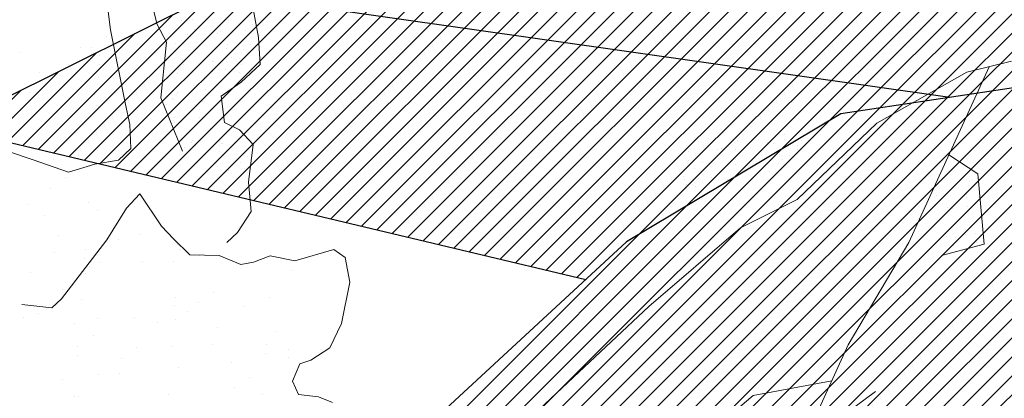
# Model space of a CAD drawing. Units: inches. Extents: x 1986 to 21484, y -1816 to 2016.
# Tile 56 of 85: x 3651.09 to 3662.33, y 1879.32 to 1883.64. Entities that reach past the tile are written whole.
import ezdxf

# ---------------------------------------------------------------- set-up
doc = ezdxf.new("R2010")
doc.units = ezdxf.units.IN
doc.layers.add('L-PLNT', color=84, linetype='Continuous', lineweight=13)
doc.layers.add('vfolhas', color=114, linetype='Continuous', lineweight=5)
doc.layers.add('vfolha2', color=110, linetype='Continuous')
doc.layers.add('vfolhas2', color=102, linetype='Continuous')
pattern_1 = [(45, (-2446.5133113, 50.986076), (-0.004419417382, 0.004419417382), [])]

# ---------------------------------------------------------------- blocks, each defined once
blk = doc.blocks.new('arbusto_PB_verde_grande')
at = {"layer": 'vfolha2'}
h = blk.add_hatch(dxfattribs=at)
h.set_pattern_fill('ANSI31', color=256, scale=0.05, style=0)
h.set_pattern_definition(pattern_1)
h.paths.add_polyline_path([(0.02944, 0.35651), (0.00028, 0.09048), (0.02625, -0.03934), (0.047, 0.06233), (0.06189, 0.09731), (0.09372, 0.26573), (0.09955, 0.43473), (0.08789, 0.61313), (0.0645, 0.72266), (0.04988, 0.6851), (0.0236, 0.51294)])
h.paths.add_polyline_path([(0.30106, 0.43789), (0.14225, 0.24871), (0.26685, 0.30022)])
h.paths.add_polyline_path([(0.37995, 0.22817), (0.23697, 0.15193), (0.18428, 0.09364), (0.11122, 0.04358), (0.02625, -0.03934), (0.28061, 0.04667), (0.36829, 0.07798), (0.46756, 0.11239), (0.61068, 0.19376), (0.71585, 0.27823), (0.55813, 0.25948)])
h.paths.add_polyline_path([(0.56101, -0.29441), (0.72752, -0.32573), (0.59024, -0.2412), (0.42962, -0.15982), (0.02625, -0.03934), (0.14922, -0.14107), (0.18838, -0.16604), (0.41501, -0.24435)])
h.paths.add_polyline_path([(-0.27429, -0.44776), (-0.30352, -0.72628), (-0.23923, -0.64175), (-0.15457, -0.45716), (0.02625, -0.03934), (-0.16328, -0.25376)])
h.paths.add_polyline_path([(-0.51963, -0.24744), (-0.67736, -0.32573), (-0.59558, -0.35072), (-0.40574, -0.32882), (-0.21007, -0.20995), (0.02625, -0.03934), (-0.14874, -0.06595), (-0.31518, -0.09101), (-0.41452, -0.15048)])
h.paths.add_polyline_path([(-0.52546, 0.25007), (-0.70947, 0.24698), (-0.51963, 0.1093), (-0.32979, 0.02167), (-0.07567, -0.0128), (-0.04234, -0.02148), (-0.35024, 0.1312)])
at = {"layer": 'vfolhas'}
h = blk.add_hatch(dxfattribs=at)
h.set_pattern_fill('ANSI31', color=256, scale=0.05, style=0)
h.set_pattern_definition(pattern_1)
h.paths.add_polyline_path([(-0.57219, 0.06233), (-0.7153, 0.10298), (-0.67736, 0.08107), (-0.62769, 0.01536), (-0.56347, -0.04095), (-0.26461, -0.0834), (-0.14874, -0.06595), (-0.10151, -0.05877), (-0.20418, -0.0472), (-0.40279, -0.00339)])
h.paths.add_polyline_path([(-0.56347, -0.04095), (-0.58279, -0.02401), (-0.72992, -0.09726), (-0.4334, -0.1679), (-0.41452, -0.15048), (-0.31518, -0.09101), (-0.26461, -0.0834)])
h.paths.add_polyline_path([(-0.2769, -0.47267), (-0.27429, -0.44776), (-0.16328, -0.25376), (0.02625, -0.03934), (-0.21007, -0.20995), (-0.2672, -0.24466), (-0.36485, -0.35697), (-0.42907, -0.46341), (-0.47586, -0.60425), (-0.37946, -0.57603)])
at = {"layer": 'vfolha2'}
for p, q in [((-0.14874, -0.06595), (-0.31518, -0.09101)), ((-0.31518, -0.09101), (-0.41452, -0.15048)), ((-0.41452, -0.15048), (-0.51963, -0.24744))]:
    blk.add_line(p, q, dxfattribs=at)
at = {"layer": 'vfolhas2'}
for p, q in [((-0.58279, -0.02401), (-0.72992, -0.09726)), ((-0.26461, -0.0834), (-0.56347, -0.04095)), ((-0.72992, -0.09726), (-0.4334, -0.1679))]:
    blk.add_line(p, q, dxfattribs=at)
blk = doc.blocks.new('PLANT-SHRUB')
for p, q in [((2172.884, 1887.124), (2174.221, 1887.672)), ((2173.498, 1887.673), (2173.023, 1887.729)), ((2170.469, 1886.715), (2170.965, 1887.348)), ((2170.965, 1887.348), (2171.41, 1887.108)), ((2173.303, 1887.296), (2174.071, 1886.806)), ((2170.958, 1887.191), (2170.958, 1887.191)), ((2171.011, 1887.275), (2171.011, 1887.275)), ((2171.008, 1887.084), (2171.008, 1887.084)), ((2171.045, 1887.117), (2171.045, 1887.117)), ((2171.149, 1887.072), (2171.149, 1887.072)), ((2171.234, 1887.125), (2171.234, 1887.125)), ((2171.581, 1886.748), (2172.884, 1887.124)), ((2171.216, 1886.993), (2171.216, 1886.993)), ((2170.81, 1886.901), (2170.81, 1886.901)), ((2169.538, 1885.91), (2171.581, 1886.748)), ((2170.636, 1886.742), (2170.636, 1886.742)), ((2170.723, 1886.795), (2170.723, 1886.795)), ((2170.753, 1886.819), (2170.753, 1886.819)), ((2170.827, 1886.781), (2170.827, 1886.781)), ((2170.946, 1886.806), (2170.946, 1886.806)), ((2170.99, 1886.76), (2170.99, 1886.76)), ((2174.071, 1886.806), (2174.764, 1886.768)), ((2170.56, 1886.329), (2170.469, 1886.715)), ((2170.599, 1886.708), (2170.599, 1886.708)), ((2170.664, 1886.627), (2170.664, 1886.627)), ((2171.072, 1886.625), (2171.072, 1886.625)), ((2170.988, 1886.571), (2170.988, 1886.571)), ((2169.31, 1886.039), (2169.765, 1885.781)), ((2169.765, 1885.781), (2170.913, 1885.503)), ((2170.913, 1885.503), (2172.174, 1885.515)), ((2172.174, 1885.515), (2172.865, 1885.309)), ((2172.865, 1885.309), (2174.246, 1885.249)), ((2174.246, 1885.249), (2175.422, 1885.249)), ((2175.422, 1885.249), (2176.598, 1885.249)), ((2171.676, 1885.061), (2171.676, 1885.061)), ((2171.748, 1885.068), (2171.748, 1885.068)), ((2171.784, 1885.103), (2171.784, 1885.103)), ((2171.888, 1885.089), (2171.888, 1885.089)), ((2171.984, 1885.074), (2171.984, 1885.074)), ((2172.051, 1885.068), (2172.051, 1885.068)), ((2172.187, 1885.064), (2172.187, 1885.064)), ((2171.773, 1884.881), (2171.773, 1884.881)), ((2171.81, 1884.915), (2171.81, 1884.915)), ((2171.934, 1884.863), (2171.934, 1884.863)), ((2172.457, 1884.857), (2172.457, 1884.857)), ((2171.975, 1884.814), (2171.975, 1884.814)), ((2172.411, 1884.739), (2172.411, 1884.739)), ((2172.597, 1884.813), (2172.597, 1884.813)), ((2172.175, 1884.679), (2172.175, 1884.679)), ((2172.294, 1884.62), (2172.294, 1884.62)), ((2172.374, 1884.705), (2172.374, 1884.705)), ((2172.714, 1884.659), (2172.714, 1884.659)), ((2172.916, 1884.619), (2172.916, 1884.619)), ((2172.175, 1884.523), (2172.175, 1884.523)), ((2172.209, 1884.566), (2172.209, 1884.566)), ((2172.242, 1884.526), (2172.242, 1884.526)), ((2172.404, 1884.504), (2172.404, 1884.504)), ((2172.832, 1884.565), (2172.832, 1884.565)), ((2172.974, 1884.53), (2172.974, 1884.53)), ((2173.011, 1884.564), (2173.011, 1884.564)), ((2172.444, 1884.472), (2172.444, 1884.472)), ((2172.676, 1884.468), (2172.676, 1884.468)), ((2172.78, 1884.455), (2172.78, 1884.455)), ((2172.942, 1884.433), (2172.942, 1884.433)), ((2172.955, 1884.474), (2172.955, 1884.474)), ((2172.436, 1884.313), (2172.436, 1884.313)), ((2172.702, 1884.274), (2172.702, 1884.274)), ((2172.776, 1884.348), (2172.776, 1884.348)), ((2177.627, 1883.579), (2177.697, 1883.42)), ((2177.697, 1883.42), (2177.847, 1883.245)), ((2177.847, 1883.245), (2177.794, 1883.087)), ((2177.22, 1883.101), (2176.932, 1882.99)), ((2177.476, 1883.057), (2177.22, 1883.101)), ((2177.598, 1883.001), (2177.476, 1883.057)), ((2177.794, 1883.087), (2177.598, 1883.001)), ((2176.932, 1882.99), (2176.543, 1882.712)), ((2176.932, 1882.99), (2176.932, 1882.99)), ((2178.147, 1882.962), (2178.147, 1882.962)), ((2177.639, 1882.854), (2177.639, 1882.854)), ((2176.543, 1882.712), (2176.387, 1882.468)), ((2177.577, 1882.788), (2177.577, 1882.788)), ((2178.12, 1882.717), (2178.12, 1882.717)), ((2178.328, 1882.689), (2178.328, 1882.689)), ((2177.726, 1882.576), (2177.726, 1882.576)), ((2177.799, 1882.644), (2177.799, 1882.644)), ((2176.387, 1882.468), (2176.42, 1882.313)), ((2177.533, 1882.548), (2177.533, 1882.548)), ((2178.154, 1882.458), (2178.154, 1882.458)), ((2176.42, 1882.313), (2176.832, 1882.102)), ((2176.926, 1882.161), (2176.926, 1882.161)), ((2177.328, 1882.212), (2177.328, 1882.212)), ((2178.171, 1882.159), (2178.171, 1882.159)), ((2178.927, 1882.225), (2178.927, 1882.225)), ((2176.832, 1882.102), (2176.998, 1881.869)), ((2177.614, 1882.084), (2177.614, 1882.084)), ((2178.002, 1882.052), (2178.002, 1882.052)), ((2178.636, 1882.089), (2178.636, 1882.089)), ((2176.998, 1881.869), (2177.187, 1881.791)), ((2177.187, 1881.791), (2177.309, 1881.713)), ((2178.529, 1881.861), (2178.529, 1881.861)), ((2177.309, 1881.713), (2177.42, 1881.469)), ((2177.309, 1881.713), (2177.309, 1881.713)), ((2177.752, 1881.731), (2177.752, 1881.731)), ((2177.96, 1881.703), (2177.96, 1881.703)), ((2178.129, 1881.688), (2178.129, 1881.688)), ((2179.175, 1881.675), (2179.175, 1881.675)), ((2178.285, 1881.66), (2178.285, 1881.66)), ((2178.827, 1881.589), (2178.827, 1881.589)), ((2179.036, 1881.561), (2179.036, 1881.561)), ((2177.42, 1881.469), (2177.66, 1881.234)), ((2178.108, 1881.475), (2178.108, 1881.475)), ((2178.182, 1881.542), (2178.182, 1881.542)), ((2178.455, 1881.545), (2178.455, 1881.545)), ((2179.36, 1881.519), (2179.36, 1881.519)), ((2179.699, 1881.543), (2179.699, 1881.543)), ((2179.731, 1881.51), (2179.731, 1881.51)), ((2176.812, 1881.351), (2176.604, 1881.085)), ((2177.088, 1881.42), (2176.812, 1881.351)), ((2177.256, 1881.42), (2177.088, 1881.42)), ((2177.589, 1881.314), (2177.589, 1881.314)), ((2177.66, 1881.234), (2177.672, 1880.972)), ((2178.611, 1881.319), (2178.611, 1881.319)), ((2179.691, 1881.28), (2179.691, 1881.28)), ((2177.848, 1881.158), (2177.848, 1881.158)), ((2179.092, 1881.156), (2179.092, 1881.156)), ((2179.309, 1881.124), (2179.309, 1881.124)), ((2179.383, 1881.192), (2179.383, 1881.192)), ((2176.604, 1881.085), (2176.269, 1880.809)), ((2177.679, 1881.051), (2177.679, 1881.051)), ((2177.71, 1881.11), (2177.71, 1881.11)), ((2178.924, 1881.049), (2178.924, 1881.049)), ((2176.53, 1880.942), (2176.53, 1880.942)), ((2177.672, 1880.972), (2177.672, 1880.772)), ((2178.104, 1880.918), (2178.104, 1880.918)), ((2179.15, 1880.905), (2179.15, 1880.905)), ((2176.269, 1880.809), (2176.269, 1880.582)), ((2176.284, 1880.801), (2176.284, 1880.801)), ((2176.411, 1880.872), (2176.411, 1880.872)), ((2176.515, 1880.858), (2176.515, 1880.858)), ((2176.678, 1880.837), (2176.678, 1880.837)), ((2176.735, 1880.717), (2176.735, 1880.717)), ((2177.672, 1880.772), (2177.597, 1880.335)), ((2177.916, 1880.674), (2177.916, 1880.674)), ((2178.912, 1880.76), (2178.912, 1880.76)), ((2176.269, 1880.582), (2176.338, 1880.404)), ((2176.517, 1880.557), (2176.517, 1880.557)), ((2176.519, 1880.553), (2176.519, 1880.553)), ((2176.561, 1880.558), (2176.561, 1880.558)), ((2176.603, 1880.606), (2176.603, 1880.606)), ((2178.234, 1880.46), (2179.071, 1880.597)), ((2178.459, 1880.603), (2178.459, 1880.603)), ((2178.667, 1880.575), (2178.667, 1880.575)), ((2179.071, 1880.597), (2179.221, 1880.597)), ((2179.221, 1880.597), (2179.446, 1880.335)), ((2176.524, 1880.524), (2176.524, 1880.524)), ((2177.822, 1880.348), (2178.234, 1880.46)), ((2178.132, 1880.544), (2178.132, 1880.544)), ((2178.234, 1880.46), (2178.234, 1880.46)), ((2178.564, 1880.441), (2178.564, 1880.441)), ((2178.586, 1880.548), (2178.586, 1880.548)), ((2178.992, 1880.532), (2178.992, 1880.532)), ((2179.376, 1880.542), (2179.376, 1880.542)), ((2179.535, 1880.461), (2179.535, 1880.461)), ((2176.338, 1880.404), (2176.16, 1880.158)), ((2176.325, 1880.342), (2176.325, 1880.342)), ((2176.331, 1880.365), (2176.331, 1880.365)), ((2176.494, 1880.344), (2176.494, 1880.344)), ((2176.758, 1880.372), (2176.758, 1880.372)), ((2177.597, 1880.335), (2177.822, 1880.348)), ((2178.49, 1880.373), (2178.49, 1880.373)), ((2176.674, 1879.698), (2176.912, 1880.313)), ((2176.745, 1880.299), (2176.745, 1880.299)), ((2176.765, 1880.308), (2176.765, 1880.308)), ((2176.869, 1880.295), (2176.869, 1880.295)), ((2175.588, 1880.197), (2175.39, 1879.961)), ((2175.884, 1880.197), (2175.588, 1880.197)), ((2175.82, 1880.107), (2175.82, 1880.107)), ((2176.16, 1880.158), (2175.884, 1880.197)), ((2176.115, 1880.149), (2176.115, 1880.149)), ((2176.442, 1880.106), (2176.442, 1880.106)), ((2176.505, 1880.172), (2176.505, 1880.172)), ((2178.079, 1880.148), (2178.079, 1880.148)), ((2178.77, 1880.155), (2178.77, 1880.155)), ((2179.125, 1880.135), (2179.125, 1880.135)), ((2175.711, 1879.991), (2175.711, 1879.991)), ((2175.735, 1880.053), (2175.735, 1880.053)), ((2176.358, 1880.052), (2176.358, 1880.052)), ((2176.752, 1880.007), (2176.752, 1880.007)), ((2178.092, 1880.009), (2178.092, 1880.009)), ((2178.601, 1880.048), (2178.601, 1880.048)), ((2175.39, 1879.961), (2175.094, 1879.497)), ((2175.505, 1879.957), (2175.505, 1879.957)), ((2175.609, 1879.943), (2175.609, 1879.943)), ((2175.771, 1879.922), (2175.771, 1879.922)), ((2175.916, 1879.967), (2175.916, 1879.967)), ((2176.043, 1879.886), (2176.043, 1879.886)), ((2176.235, 1879.985), (2176.235, 1879.985)), ((2176.715, 1879.974), (2176.715, 1879.974)), ((2176.746, 1879.987), (2176.746, 1879.987)), ((2177.321, 1879.888), (2177.141, 1879.678)), ((2177.511, 1879.888), (2177.321, 1879.888)), ((2177.741, 1879.738), (2177.511, 1879.888)), ((2175.339, 1879.801), (2175.339, 1879.801)), ((2175.441, 1879.804), (2175.441, 1879.804)), ((2175.705, 1879.774), (2175.705, 1879.774)), ((2175.742, 1879.807), (2175.742, 1879.807)), ((2175.952, 1879.806), (2175.952, 1879.806)), ((2175.962, 1879.8), (2175.962, 1879.8)), ((2176.147, 1879.872), (2176.147, 1879.872)), ((2176.309, 1879.851), (2176.309, 1879.851)), ((2176.492, 1879.787), (2176.492, 1879.787)), ((2176.516, 1879.791), (2176.516, 1879.791)), ((2176.581, 1879.815), (2176.581, 1879.815)), ((2176.584, 1879.799), (2176.584, 1879.799)), ((2176.685, 1879.801), (2176.685, 1879.801)), ((2178.561, 1879.778), (2178.561, 1879.778)), ((2176.19, 1879.28), (2176.674, 1879.698)), ((2177.141, 1879.678), (2177.02, 1879.478)), ((2178.021, 1879.598), (2177.741, 1879.738)), ((2175.506, 1879.591), (2175.506, 1879.591)), ((2175.574, 1879.553), (2175.574, 1879.553)), ((2175.658, 1879.607), (2175.658, 1879.607)), ((2175.699, 1879.606), (2175.699, 1879.606)), ((2176.196, 1879.552), (2176.196, 1879.552)), ((2176.222, 1879.599), (2176.222, 1879.599)), ((2176.28, 1879.606), (2176.28, 1879.606)), ((2176.306, 1879.598), (2176.306, 1879.598)), ((2176.343, 1879.632), (2176.343, 1879.632)), ((2177.809, 1879.543), (2177.809, 1879.543)), ((2178.021, 1879.598), (2178.021, 1879.598)), ((2178.221, 1879.219), (2178.021, 1879.598)), ((2178.091, 1879.616), (2178.091, 1879.616)), ((2178.299, 1879.589), (2178.299, 1879.589)), ((2178.623, 1879.546), (2178.623, 1879.546)), ((2177.02, 1879.478), (2176.561, 1878.739)), ((2177.02, 1879.478), (2177.02, 1879.478)), ((2175.859, 1879.393), (2175.859, 1879.393)), ((2175.94, 1879.421), (2175.94, 1879.421)), ((2175.963, 1879.379), (2175.963, 1879.379)), ((2176.107, 1879.416), (2176.107, 1879.416)), ((2176.125, 1879.358), (2176.125, 1879.358)), ((2178.054, 1879.378), (2178.054, 1879.378)), ((2175.8, 1879.3), (2175.8, 1879.3)), ((2175.896, 1879.223), (2175.896, 1879.223)), ((2175.933, 1879.257), (2175.933, 1879.257)), ((2176.131, 1879.063), (2176.19, 1879.28)), ((2177.273, 1879.258), (2177.273, 1879.258)), ((2178.221, 1879.219), (2178.221, 1879.219)), ((2178.361, 1878.959), (2178.221, 1879.219)), ((2176.119, 1879.105), (2176.119, 1879.105)), ((2177.202, 1879.157), (2177.202, 1879.157)), ((2175.884, 1878.61), (2176.131, 1879.063)), ((2177.034, 1879.049), (2177.034, 1879.049)), ((2177.513, 1879.003), (2177.513, 1879.003)), ((2176.852, 1878.872), (2176.852, 1878.872)), ((2176.926, 1878.94), (2176.926, 1878.94)), ((2176.646, 1878.772), (2176.646, 1878.772)), ((2176.561, 1878.739), (2176.437, 1878.57)), ((2176.854, 1878.744), (2176.854, 1878.744)), ((2176.949, 1878.647), (2176.949, 1878.647)), ((2177.179, 1878.701), (2177.179, 1878.701)), ((2177.486, 1878.542), (2177.486, 1878.542)), ((2177.722, 1878.63), (2177.722, 1878.63)), ((2177.488, 1878.233), (2177.488, 1878.233))]:
    blk.add_line(p, q)

msp = doc.modelspace()

# ---------------------------------------------------------------- block references
at = {"layer": 'L-PLNT', "rotation": 223.1883365522388}
msp.add_blockref('PLANT-SHRUB', (3953.27, 4742.965), dxfattribs=at)
at = {"layer": 'L-PLNT', "xscale": 24.60366729364114, "yscale": 24.60366729364114, "zscale": 24.60366729364114}
msp.add_blockref('arbusto_PB_verde_grande', (3668.218, 1884.805), dxfattribs=at)

doc.saveas('drawing.dxf')
